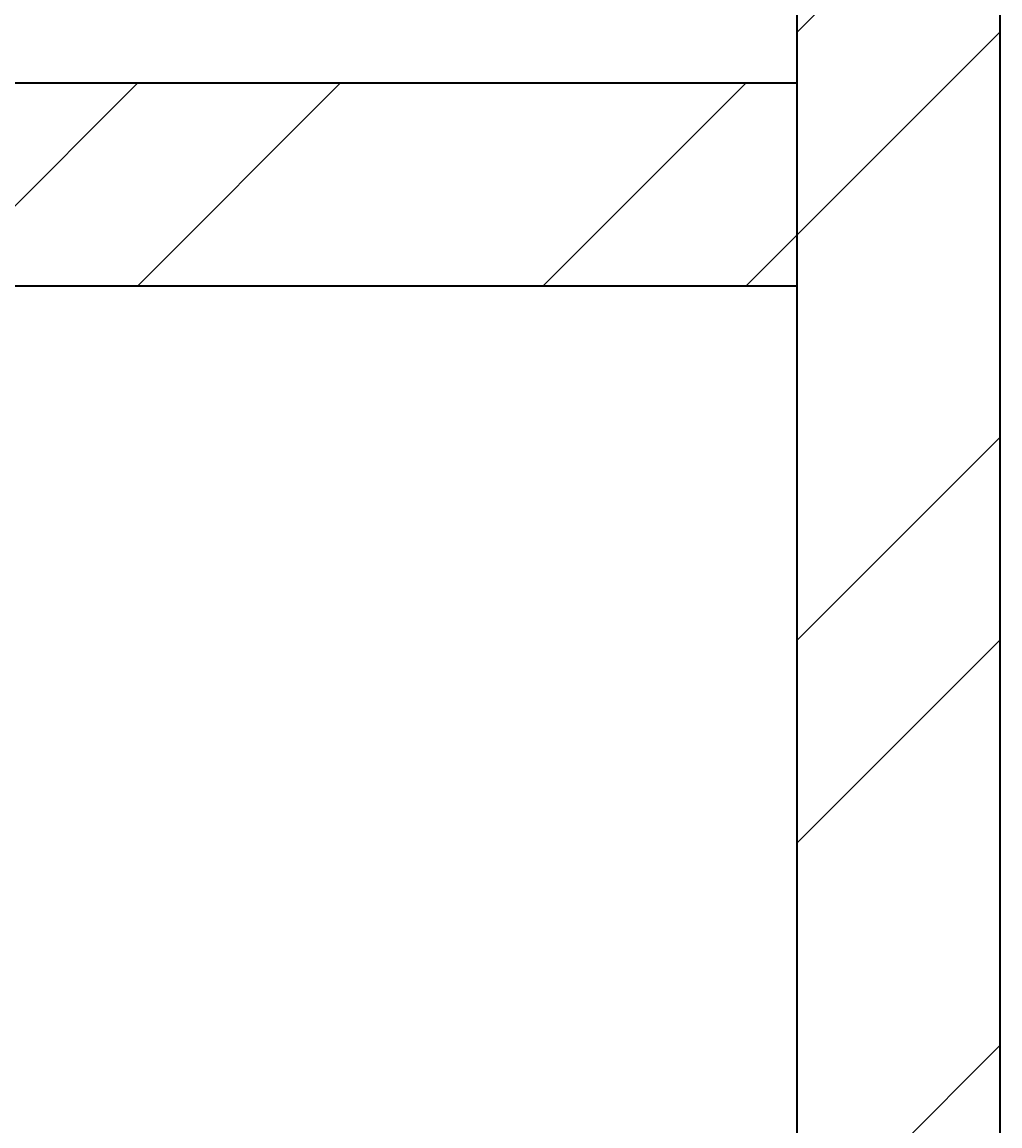
# Model space of a CAD drawing. Units: inches. Extents: x 1962 to 2771, y 1245 to 2660.
# Tile 81 of 114: x 2639 to 2661, y 2107 to 2131. Entities that reach past the tile are written whole.
import ezdxf

# ---------------------------------------------------------------- set-up
doc = ezdxf.new("R2010")
doc.units = ezdxf.units.IN
for name, color, linetype, lineweight in [('A-ANNO-DIMS', 2, 'Continuous', 18), ('A-WALL', 7, 'Continuous', 35), ('A-WALL-PATT', 252, 'Continuous', 13)]:
    doc.layers.add(name, color=color, linetype=linetype, lineweight=lineweight)
doc.styles.get("Standard").update_dxf_attribs({"font": 'arial.ttf'})
doc.dimstyles.get("Standard").update_dxf_attribs({"dimtxt": 0.18, "dimasz": 0.18, "dimexe": 0.18, "dimexo": 0.0625, "dimgap": 0.09, "dimtad": 0, "dimtih": 1, "dimtoh": 1, "dimdec": 4, "dimzin": 0, "dimdsep": 46, "dimtxsty": 'Standard', "dimcen": 0.09, "dimadec": 0, "dimazin": 0, "dimtfac": 1, "dimtdec": 4, "dimtofl": 0, "dimtmove": 0, "dimatfit": 3, "dimfxl": 1, "dimtolj": 1, "dimtzin": 0, "dimarcsym": 0})

# ---------------------------------------------------------------- blocks, each defined once
blk = doc.blocks.new('*D40')
at = {"layer": 'A-ANNO-DIMS', "color": 0, "lineweight": -2, "transparency": 16777216}
for p, q in [((2072.02, 2033.906), (2072.02, 2583.474)), ((2660.807, 2524.406), (2660.807, 2583.474)), ((2072.2, 2583.294), (2366.02, 2583.294)), ((2660.627, 2583.294), (2366.808, 2583.294))]:
    blk.add_line(p, q, dxfattribs=at)
at = {"layer": 'A-ANNO-DIMS', "color": 0, "transparency": 16777216}
for points in [[(2072.2, 2583.324), (2072.2, 2583.264), (2072.02, 2583.294)], [(2660.627, 2583.324), (2660.627, 2583.264), (2660.807, 2583.294)]]:
    blk.add_solid(points, dxfattribs=at)
at = {"layer": 'Defpoints', "color": 0, "transparency": 16777216}
for p in [(2660.807, 2583.294), (2660.807, 2524.344), (2072.02, 2033.844)]:
    blk.add_point(p, dxfattribs=at)
at = {"layer": 'A-ANNO-DIMS', "color": 0, "transparency": 16777216, "insert": (2366.414, 2583.294), "char_height": 0.18, "attachment_point": 5}
blk.add_mtext('\\A1;588.8', dxfattribs=at)

msp = doc.modelspace()

# ---------------------------------------------------------------- hatches: boundary and pattern name
at = {"layer": 'A-WALL-PATT'}
h = msp.add_hatch(dxfattribs=at)
h.set_pattern_fill('ANSI32', color=256)
h.paths.add_polyline_path([(2090.8074, 2467.3437), (2141.6481, 2467.3437), (2141.6481, 2469.5937), (2141.6481, 2471.8437), (2086.3074, 2471.8437), (2086.3074, 2422.5333), (2090.8074, 2422.5333)])
h.paths.add_polyline_path([(2282.7664, 2471.8437), (2204.8982, 2471.8437), (2204.8982, 2467.3437), (2234.8074, 2467.3437), (2234.8074, 2311.3437), (2228.7492, 2311.3437), (2228.7492, 2306.8437), (2234.8074, 2306.8437), (2331.9227, 2306.8437), (2331.9227, 2309.0937), (2331.9227, 2311.3437), (2239.3074, 2311.3437), (2239.3074, 2467.3437), (2282.7664, 2467.3437), (2282.7664, 2469.5937)])
h.paths.add_polyline_path([(2471.4531, 2519.8437), (2552.011, 2519.8437), (2564.3996, 2519.8437), (2564.3996, 2511.1389), (2568.8996, 2511.1389), (2568.8996, 2524.3437), (2466.9531, 2524.3437), (2466.9531, 2471.8437), (2450.0749, 2471.8437), (2446.4672, 2471.8437), (2446.4672, 2467.3437), (2450.0749, 2467.3437), (2475.9988, 2467.3437), (2475.9988, 2469.5937), (2475.9988, 2471.8437), (2471.4531, 2471.8437)])
h.paths.add_polyline_path([(2575.2231, 2469.5937), (2575.2231, 2471.8437), (2568.8996, 2471.8437), (2568.8996, 2487.1389), (2564.3996, 2487.1389), (2564.3996, 2471.8437), (2556.511, 2471.8437), (2499.2904, 2471.8437), (2499.2904, 2467.3437), (2507.8074, 2467.3437), (2507.8074, 2311.3437), (2414.863, 2311.3437), (2414.863, 2306.8437), (2512.3074, 2306.8437), (2517.0114, 2306.8437), (2517.0114, 2309.0937), (2517.0114, 2311.3437), (2512.3074, 2311.3437), (2512.3074, 2467.3437), (2575.2231, 2467.3437)])
h.paths.add_polyline_path([(2660.8074, 2471.8437), (2600.9602, 2471.8437), (2600.9602, 2467.3437), (2656.3074, 2467.3437), (2656.3074, 2432.5704), (2660.8074, 2432.5704)])
h.paths.add_polyline_path([(2660.8074, 2372.5704), (2656.3074, 2372.5704), (2656.3074, 2311.3437), (2600.276, 2311.3437), (2600.276, 2309.0937), (2600.276, 2306.8437), (2656.3074, 2306.8437), (2656.3074, 2296.2593), (2660.8074, 2296.2593)])
h.paths.add_polyline_path([(2572.3074, 2306.8437), (2577.1385, 2306.8437), (2577.1385, 2311.3437), (2551.082, 2311.3437), (2551.082, 2306.8437), (2567.8074, 2306.8437), (2567.8074, 2258.8437), (2540.0574, 2258.8437), (2540.0574, 2256.5937), (2540.0574, 2254.3437), (2567.8074, 2254.3437), (2656.3074, 2254.3437), (2656.3074, 2236.9085), (2660.8074, 2236.9085), (2660.8074, 2272.2593), (2656.3074, 2272.2593), (2656.3074, 2258.8437), (2572.3074, 2258.8437)])
h.paths.add_polyline_path([(2512.3074, 2254.3437), (2518.8716, 2254.3437), (2518.8716, 2256.5937), (2518.8716, 2258.8437), (2507.8074, 2258.8437), (2507.8074, 2177.8437), (2567.8074, 2177.8437), (2567.8074, 2172.9628), (2572.3074, 2172.9628), (2572.3074, 2177.8437), (2656.3074, 2177.8437), (2656.3074, 2166.4846), (2660.8074, 2166.4846), (2660.8074, 2200.9085), (2656.3074, 2200.9085), (2656.3074, 2182.3437), (2512.3074, 2182.3437)])
h.paths.add_polyline_path([(2656.3074, 2129.8437), (2572.3074, 2129.8437), (2572.3074, 2150.3044), (2570.0574, 2150.3044), (2567.8074, 2150.3044), (2567.8074, 2129.8437), (2507.8074, 2129.8437), (2507.8074, 2116.3027), (2510.0574, 2116.3027), (2512.3074, 2116.3027), (2512.3074, 2125.3437), (2567.8074, 2125.3437), (2572.3074, 2125.3437), (2656.3074, 2125.3437)])
h.paths.add_polyline_path([(2090.8074, 2362.5333), (2086.3074, 2362.5333), (2086.3074, 2298.6242), (2090.8074, 2298.6242), (2090.8074, 2306.8437), (2174.8074, 2306.8437), (2174.8074, 2286.4178), (2179.3074, 2286.4178), (2179.3074, 2306.8437), (2192.8641, 2306.8437), (2192.8641, 2309.0937), (2192.8641, 2311.3437), (2090.8074, 2311.3437)])
h.paths.add_polyline_path([(2209.156, 2258.8437), (2179.3074, 2258.8437), (2179.3074, 2263.2236), (2177.0574, 2263.2236), (2174.8074, 2263.2236), (2174.8074, 2258.8437), (2090.8074, 2258.8437), (2090.8074, 2274.6242), (2086.3074, 2274.6242), (2086.3074, 2238.2967), (2088.5574, 2238.2967), (2090.8074, 2238.2967), (2090.8074, 2254.3437), (2209.156, 2254.3437)])
h.paths.add_polyline_path([(2090.8074, 2177.8437), (2234.8074, 2177.8437), (2234.8074, 2173.1428), (2239.3074, 2173.1428), (2239.3074, 2258.8437), (2230.8442, 2258.8437), (2230.8442, 2256.5937), (2230.8442, 2254.3437), (2234.8074, 2254.3437), (2234.8074, 2182.3437), (2090.8074, 2182.3437), (2090.8074, 2202.2967), (2086.3074, 2202.2967), (2086.3074, 2140.0389), (2090.8074, 2140.0389)])
h.paths.add_polyline_path([(2090.8074, 2080.0389), (2086.3074, 2080.0389), (2086.3074, 2033.8437), (2090.8074, 2033.8437)], flags=17)
h.paths.add_polyline_path([(2244.9405, 2033.8437), (2239.3074, 2033.8437), (2239.3074, 2142.0665), (2237.2592, 2142.0665), (2234.8074, 2142.0665), (2234.8074, 2033.8437), (2090.8074, 2033.8437), (2076.5204, 2033.8437), (2072.0204, 2033.8437), (2072.0204, 2000.4493), (2076.5204, 2000.4493), (2076.5204, 2029.3437), (2090.8074, 2029.3437), (2244.9405, 2029.3437), (2244.9405, 2031.5937)])
h.paths.add_polyline_path([(2234.8074, 1933.3437), (2076.5204, 1933.3437), (2076.5204, 1952.4493), (2074.2704, 1952.4493), (2072.0204, 1952.4493), (2072.0204, 1933.3437), (2072.0204, 1928.8437), (2234.8074, 1928.8437)])
h.paths.add_polyline_path([(2090.8074, 1928.8437), (2086.3074, 1928.8437), (2086.3074, 1906.5013), (2090.8074, 1906.5013)])
h.paths.add_polyline_path([(2090.8074, 1846.5013), (2086.3074, 1846.5013), (2086.3074, 1769.9917), (2088.5574, 1769.9917), (2090.8074, 1769.9917), (2090.8074, 1780.3437), (2234.8074, 1780.3437), (2234.8074, 1708.3437), (2230.3764, 1708.3437), (2230.3764, 1703.8437), (2239.3074, 1703.8437), (2239.3074, 1792.6669), (2237.0574, 1792.6669), (2234.8074, 1792.6669), (2234.8074, 1784.8437), (2090.8074, 1784.8437)])
h.paths.add_polyline_path([(2239.3074, 1928.8437), (2244.9405, 1928.8437), (2244.9405, 1931.0937), (2244.9405, 1933.3437), (2234.8074, 1933.3437), (2234.8074, 1928.8437), (2234.8074, 1825.5949), (2239.3074, 1825.5949)])
h.paths.add_polyline_path([(2148.0425, 1649.0937), (2148.0425, 1651.3437), (2090.8074, 1651.3437), (2090.8074, 1646.8437), (2148.0425, 1646.8437)], flags=0)
h.paths.add_polyline_path([(2207.5601, 1708.3437), (2090.8074, 1708.3437), (2090.8074, 1703.8437), (2174.8074, 1703.8437), (2174.8074, 1651.3437), (2170.4457, 1651.3437), (2170.4457, 1646.8437), (2195.9924, 1646.8437), (2195.9924, 1649.0937), (2195.9924, 1651.3437), (2179.3074, 1651.3437), (2179.3074, 1703.8437), (2207.5601, 1703.8437), (2207.5601, 1706.0937)])
h.paths.add_polyline_path([(2090.8074, 1733.9917), (2086.3074, 1733.9917), (2086.3074, 1696.1032), (2088.5574, 1696.1032), (2090.8074, 1696.1032)])
h.paths.add_polyline_path([(2090.8074, 1672.1032), (2086.3074, 1672.1032), (2086.3074, 1600.3335), (2090.8074, 1600.3335)])
h.paths.add_polyline_path([(2090.8074, 1540.3335), (2086.3074, 1540.3335), (2086.3074, 1486.3437), (2139.6766, 1486.3437), (2139.6766, 1490.8437), (2090.8074, 1490.8437)])
h.paths.add_polyline_path([(2302.3876, 1490.8437), (2239.3074, 1490.8437), (2239.3074, 1646.8437), (2335.9994, 1646.8437), (2335.9994, 1651.3437), (2229.884, 1651.3437), (2229.884, 1646.8437), (2234.8074, 1646.8437), (2234.8074, 1490.8437), (2202.7103, 1490.8437), (2202.7103, 1488.5937), (2202.7103, 1486.3437), (2275.0699, 1486.3437), (2275.0699, 1475.772), (2279.5699, 1475.772), (2279.5699, 1486.3437), (2302.3876, 1486.3437)])
h.paths.add_polyline_path([(2279.5699, 1451.772), (2275.0699, 1451.772), (2275.0699, 1438.3437), (2174.8074, 1438.3437), (2174.8074, 1486.3437), (2179.7922, 1486.3437), (2179.7922, 1490.8437), (2163.3585, 1490.8437), (2163.3585, 1488.5937), (2163.3585, 1486.3437), (2170.3074, 1486.3437), (2170.3074, 1433.8437), (2279.5699, 1433.8437)])
h.paths.add_polyline_path([(2427.2363, 1490.8437), (2375.8074, 1490.8437), (2375.8074, 1646.8437), (2381.6401, 1646.8437), (2381.6401, 1651.3437), (2365.887, 1651.3437), (2365.887, 1649.0937), (2365.887, 1646.8437), (2371.3074, 1646.8437), (2371.3074, 1490.8437), (2327.5627, 1490.8437), (2327.5627, 1488.5937), (2327.5627, 1486.3437), (2371.3074, 1486.3437), (2371.3074, 1433.8437), (2375.8074, 1433.8437), (2375.8074, 1486.3437), (2427.2363, 1486.3437)])
h.paths.add_polyline_path([(2512.3074, 1646.8437), (2519.4351, 1646.8437), (2519.4351, 1649.0937), (2519.4351, 1651.3437), (2507.8074, 1651.3437), (2416.0063, 1651.3437), (2416.0063, 1649.0937), (2416.0063, 1646.8437), (2507.8074, 1646.8437), (2507.8074, 1490.8437), (2497.0532, 1490.8437), (2497.0532, 1488.5937), (2497.0532, 1486.3437), (2574.9344, 1486.3437), (2574.9344, 1476.0181), (2579.4344, 1476.0181), (2579.4344, 1486.3437), (2584.4872, 1486.3437), (2584.3074, 1490.8437), (2512.3074, 1490.8437)])
h.paths.add_polyline_path([(2470.5091, 1486.3437), (2473.9767, 1486.3437), (2473.9767, 1490.8437), (2449.6605, 1490.8437), (2449.6605, 1488.5937), (2449.6605, 1486.3437), (2466.0091, 1486.3437), (2466.0091, 1433.8437), (2470.5091, 1433.8437), (2579.4344, 1433.8437), (2579.4344, 1452.0181), (2574.9344, 1452.0181), (2574.9344, 1438.3437), (2554.5091, 1438.3437), (2470.5091, 1438.3437)])
h.paths.add_polyline_path([(2656.3074, 1490.8437), (2611.86, 1490.8437), (2611.86, 1486.3437), (2656.3074, 1486.3437)])
h.paths.add_polyline_path([(2660.8074, 1532.7007), (2658.5574, 1532.7007), (2656.3074, 1532.7007), (2656.3074, 1486.3437), (2660.8074, 1486.3437)])
h.paths.add_polyline_path([(2660.8074, 1664.9663), (2656.3074, 1664.9663), (2656.3074, 1651.3437), (2602.2313, 1651.3437), (2602.2313, 1646.8437), (2656.3074, 1646.8437), (2656.3074, 1592.7007), (2660.8074, 1592.7007)])
h.paths.add_polyline_path([(2660.8074, 1724.5221), (2656.3074, 1724.5221), (2656.3074, 1703.8437), (2542.4725, 1703.8437), (2542.4725, 1699.3437), (2567.8074, 1699.3437), (2567.8074, 1651.3437), (2552.7766, 1651.3437), (2552.7766, 1649.0937), (2552.7766, 1646.8437), (2577.2878, 1646.8437), (2577.2878, 1649.0937), (2577.2878, 1651.3437), (2572.3074, 1651.3437), (2572.3074, 1699.3437), (2656.3074, 1699.3437), (2656.3074, 1688.9663), (2660.8074, 1688.9663)])
h.paths.add_polyline_path([(2660.8074, 1880.6524), (2656.3074, 1880.6524), (2656.3074, 1832.8437), (2512.3074, 1832.8437), (2512.3074, 1837.8959), (2507.8074, 1837.8959), (2507.8074, 1828.3437), (2567.8074, 1828.3437), (2567.8074, 1804.3437), (2572.3074, 1804.3437), (2572.3074, 1828.3437), (2656.3074, 1828.3437), (2656.3074, 1818.6778), (2660.8074, 1818.6778)])
h.paths.add_polyline_path([(2660.8074, 1794.6778), (2656.3074, 1794.6778), (2656.3074, 1780.3437), (2572.3074, 1780.3437), (2572.3074, 1783.0303), (2570.0574, 1783.0303), (2567.8074, 1783.0303), (2567.8074, 1780.3437), (2507.8074, 1780.3437), (2507.8074, 1699.3437), (2517.8858, 1699.3437), (2517.8858, 1701.5937), (2517.8858, 1703.8437), (2512.3074, 1703.8437), (2512.3074, 1775.8437), (2656.3074, 1775.8437), (2656.3074, 1760.5221), (2660.8074, 1760.5221)])
h.paths.add_polyline_path([(2660.8074, 1981.3437), (2660.8074, 2020.2808), (2658.5574, 2020.2808), (2656.3074, 2020.2808), (2656.3074, 1981.3437), (2512.3074, 1981.3437), (2512.3074, 2086.6996), (2507.8074, 2086.6996), (2507.8074, 1981.3437), (2375.8074, 1981.3437), (2375.8074, 1986.8505), (2373.5574, 1986.8505), (2371.3074, 1986.8505), (2371.3074, 1973.2607), (2375.8074, 1973.2607), (2375.8074, 1976.8437), (2507.8074, 1976.8437), (2507.8074, 1865.4281), (2510.0574, 1865.4281), (2512.3074, 1865.4281), (2512.3074, 1976.8437), (2660.8074, 1976.8437)])
h.paths.add_polyline_path([(2375.8074, 1940.297), (2373.5574, 1940.297), (2371.3074, 1940.297), (2371.3074, 1933.3437), (2278.4434, 1933.3437), (2278.4434, 1928.8437), (2371.3074, 1928.8437), (2371.3074, 1651.3437), (2375.8074, 1651.3437)])
h.paths.add_polyline_path([(2660.8074, 1976.8437), (2656.3074, 1976.8437), (2656.3074, 1940.6524), (2660.8074, 1940.6524)], flags=17)
h.paths.add_polyline_path([(2660.8074, 2142.4846), (2656.3074, 2142.4846), (2656.3074, 2080.2808), (2660.8074, 2080.2808)])
h.paths.add_polyline_path([(2381.4189, 2311.3437), (2375.8074, 2311.3437), (2375.8074, 2467.3437), (2424.7242, 2467.3437), (2424.7242, 2469.5937), (2424.7242, 2471.8437), (2375.8074, 2471.8437), (2375.8074, 2524.3437), (2371.3074, 2524.3437), (2371.3074, 2471.8437), (2307.2097, 2471.8437), (2307.2097, 2467.3437), (2371.3074, 2467.3437), (2371.3074, 2311.3437), (2366.8901, 2311.3437), (2366.8901, 2306.8437), (2371.3074, 2306.8437), (2371.3074, 2033.8437), (2279.6589, 2033.8437), (2279.6589, 2029.3437), (2371.3074, 2029.3437), (2371.3074, 2014.2598), (2375.8074, 2014.2598), (2375.8074, 2306.8437), (2381.4189, 2306.8437)])
h.paths.add_polyline_path([(2263.3074, 2524.3437), (2170.3074, 2524.3437), (2170.3074, 2519.8437), (2170.3074, 2471.8437), (2165.0312, 2471.8437), (2165.0312, 2467.3437), (2179.6721, 2467.3437), (2179.6721, 2469.5161), (2179.6721, 2471.8437), (2174.8074, 2471.8437), (2174.8074, 2519.8437), (2258.8074, 2519.8437), (2258.8074, 2511.6436), (2263.3074, 2511.6436)])
h.paths.add_polyline_path([(2245.0232, 1361.4123), (2492.9468, 1361.4123), (2492.9468, 1398.505), (2245.0232, 1398.505)], flags=9)
h.paths.add_polyline_path([(2388.1434, 2086.6936), (2425.0704, 2086.6936), (2425.0704, 2105.3509), (2388.1434, 2105.3509)], flags=9)
h.paths.add_polyline_path([(2404.922, 2242.6744), (2445.7337, 2242.6744), (2445.7337, 2261.3318), (2404.922, 2261.3318)], flags=9)
h.paths.add_polyline_path([(2269.4107, 2156.7935), (2306.3378, 2156.7935), (2306.3378, 2175.4508), (2269.4107, 2175.4508)], flags=9)
h.paths.add_polyline_path([(2269.3277, 2233.4343), (2306.2547, 2233.4343), (2306.2547, 2252.0917), (2269.3277, 2252.0917)], flags=9)
h.paths.add_polyline_path([(2431.6052, 2320.6922), (2470.4456, 2320.6922), (2470.4456, 2339.3495), (2431.6052, 2339.3495)], flags=25)
h.paths.add_polyline_path([(2249.6902, 2315.7608), (2288.5306, 2315.7608), (2288.5306, 2334.4182), (2249.6902, 2334.4182)], flags=25)
h.paths.add_polyline_path([(2096.9301, 2314.3181), (2135.7704, 2314.3181), (2135.7704, 2332.9755), (2096.9301, 2332.9755)], flags=25)
h.paths.add_polyline_path([(2134.3475, 2285.7089), (2161.4655, 2285.7089), (2161.4655, 2304.3662), (2134.3475, 2304.3662)], flags=9)
h.paths.add_polyline_path([(2126.5155, 2209.4076), (2159.9227, 2209.4076), (2159.9227, 2228.065), (2126.5155, 2228.065)], flags=25)
h.paths.add_polyline_path([(2110.5753, 2141.5299), (2149.4157, 2141.5299), (2149.4157, 2160.1872), (2110.5753, 2160.1872)], flags=25)
h.paths.add_polyline_path([(2249.8618, 1968.3317), (2286.3966, 1968.3317), (2286.3966, 1986.989), (2249.8618, 1986.989)], flags=9)
h.paths.add_polyline_path([(2395.9507, 1777.0051), (2436.7624, 1777.0051), (2436.7624, 1795.6625), (2395.9507, 1795.6625)], flags=9)
h.paths.add_polyline_path([(2398.5259, 1888.5651), (2435.0062, 1888.5651), (2435.0062, 1907.2224), (2398.5259, 1907.2224)], flags=25)
h.paths.add_polyline_path([(2259.3506, 1728.3559), (2296.2776, 1728.3559), (2296.2776, 1747.0132), (2259.3506, 1747.0132)], flags=9)
h.paths.add_polyline_path([(2271.3698, 1845.268), (2308.2968, 1845.268), (2308.2968, 1863.9253), (2271.3698, 1863.9253)], flags=9)
h.paths.add_polyline_path([(2120.9355, 1786.3027), (2159.7759, 1786.3027), (2159.7759, 1804.9601), (2120.9355, 1804.9601)], flags=25)
h.paths.add_polyline_path([(2121.3164, 1732.1043), (2154.7236, 1732.1043), (2154.7236, 1750.7616), (2121.3164, 1750.7616)], flags=25)
h.paths.add_polyline_path([(2118.3706, 1678.8997), (2147.5282, 1678.8997), (2147.5282, 1697.557), (2118.3706, 1697.557)], flags=25)
h.paths.add_polyline_path([(2385.9227, 1493.557), (2424.763, 1493.557), (2424.763, 1512.2143), (2385.9227, 1512.2143)], flags=25)
h.paths.add_polyline_path([(2248.7058, 1500.0256), (2287.5462, 1500.0256), (2287.5462, 1518.6829), (2248.7058, 1518.6829)], flags=25)
h.paths.add_polyline_path([(2104.1669, 1617.3771), (2143.0073, 1617.3771), (2143.0073, 1636.0344), (2104.1669, 1636.0344)], flags=9)
h.paths.add_polyline_path([(2096.0714, 1447.8824), (2137.3845, 1447.8824), (2137.3845, 1458.1859), (2096.0714, 1458.1859)], flags=9)
h.paths.add_polyline_path([(2180.6114, 1440.325), (2209.7689, 1440.325), (2209.7689, 1458.9823), (2180.6114, 1458.9823)], flags=25)
h.paths.add_polyline_path([(2316.1698, 1447.9637), (2357.4829, 1447.9637), (2357.4829, 1458.2673), (2316.1698, 1458.2673)], flags=9)
h.paths.add_polyline_path([(2397.6187, 1447.9637), (2438.9318, 1447.9637), (2438.9318, 1458.2673), (2397.6187, 1458.2673)], flags=9)
h.paths.add_polyline_path([(2473.0778, 1439.5953), (2502.2354, 1439.5953), (2502.2354, 1458.2527), (2473.0778, 1458.2527)], flags=25)
h.paths.add_polyline_path([(2589.7027, 1447.8819), (2631.0158, 1447.8819), (2631.0158, 1458.1855), (2589.7027, 1458.1855)], flags=9)
h.paths.add_polyline_path([(2522.4009, 1497.5285), (2561.2413, 1497.5285), (2561.2413, 1516.1859), (2522.4009, 1516.1859)], flags=25)
h.paths.add_polyline_path([(2579.6565, 1671.3482), (2608.8141, 1671.3482), (2608.8141, 1690.0056), (2579.6565, 1690.0056)], flags=25)
h.paths.add_polyline_path([(2544.7038, 1725.5064), (2578.1111, 1725.5064), (2578.1111, 1744.1637), (2544.7038, 1744.1637)], flags=25)
h.paths.add_polyline_path([(2578.1191, 1807.472), (2607.2766, 1807.472), (2607.2766, 1826.1293), (2578.1191, 1826.1293)], flags=25)
h.paths.add_polyline_path([(2595.0614, 1835.1839), (2633.9018, 1835.1839), (2633.9018, 1853.8413), (2595.0614, 1853.8413)], flags=25)
h.paths.add_polyline_path([(2567.0097, 2097.7035), (2605.8501, 2097.7035), (2605.8501, 2116.3609), (2567.0097, 2116.3609)], flags=9)
h.paths.add_polyline_path([(2586.644, 2134.6454), (2615.8015, 2134.6454), (2615.8015, 2153.3027), (2586.644, 2153.3027)], flags=9)
h.paths.add_polyline_path([(2544.6185, 2212.6783), (2578.0258, 2212.6783), (2578.0258, 2231.3356), (2544.6185, 2231.3356)], flags=25)
h.paths.add_polyline_path([(2577.0273, 2256.9023), (2606.1849, 2256.9023), (2606.1849, 2275.5597), (2577.0273, 2275.5597)], flags=24)
h.paths.add_polyline_path([(2605.2683, 2315.2821), (2644.1087, 2315.2821), (2644.1087, 2333.9395), (2605.2683, 2333.9395)], flags=25)
h.paths.add_polyline_path([(2583.1244, 2496.1815), (2624.4375, 2496.1815), (2624.4375, 2506.4851), (2583.1244, 2506.4851)], flags=9)
h.paths.add_polyline_path([(2474.761, 2497.0823), (2503.9185, 2497.0823), (2503.9185, 2515.7397), (2474.761, 2515.7397)], flags=25)
h.paths.add_polyline_path([(2387.5787, 2494.2563), (2428.902, 2494.2563), (2428.902, 2504.5598), (2387.5787, 2504.5598)], flags=9)
h.paths.add_polyline_path([(2300.1657, 2500.1564), (2341.4788, 2500.1564), (2341.4788, 2510.46), (2300.1657, 2510.46)], flags=25)
h.paths.add_polyline_path([(2176.8589, 2497.5843), (2206.0165, 2497.5843), (2206.0165, 2516.2416), (2176.8589, 2516.2416)], flags=25)
h.paths.add_polyline_path([(2097.4668, 2494.9762), (2138.7799, 2494.9762), (2138.7799, 2505.2798), (2097.4668, 2505.2798)], flags=9)

# ---------------------------------------------------------------- linework, layer by layer
at = {"layer": 'A-WALL'}
for p, q in [((2660.8074, 2471.8437), (2660.8074, 1976.8437)), ((2656.3074, 2177.8437), (2656.3074, 1981.3437)), ((2572.3074, 2129.8437), (2656.3074, 2129.8437)), ((2656.3074, 2129.8437), (2656.3074, 2125.3437)), ((2656.3074, 2125.3437), (2572.3074, 2125.3437))]:
    msp.add_line(p, q, dxfattribs=at)

# ---------------------------------------------------------------- dimensions: what is measured, and where the dimension line sits
at = {"layer": 'A-ANNO-DIMS'}
dim = msp.add_linear_dim(base=(2660.8074, 2583.2937), p1=(2072.0204, 2033.8437), p2=(2660.8074, 2524.3437), dimstyle='Standard', override={"dimdec": 1, "dimlfac": 1, "dimrnd": 0, "dimzin": 0, "dimdsep": 46, "dimlunit": 2}, dxfattribs=at)
dim.commit()
dim.dimension.update_dxf_attribs({"geometry": '*D40', "text_midpoint": (2366.4139, 2583.2937)})

doc.saveas('drawing.dxf')
